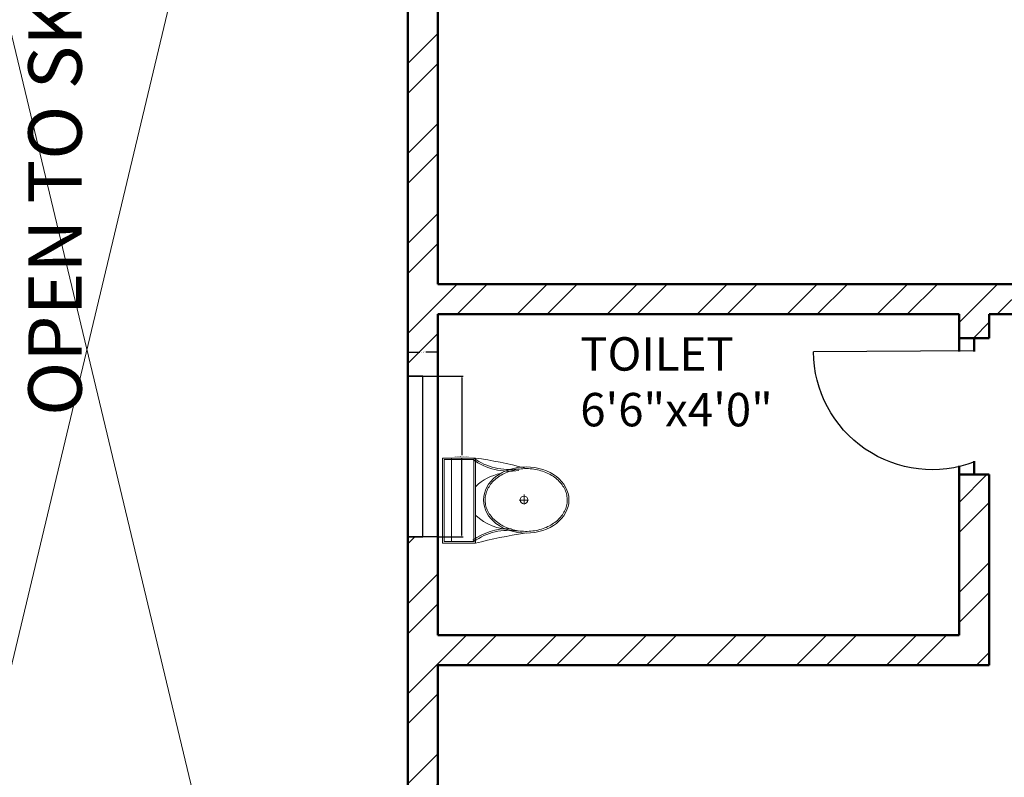
# Model space of a CAD drawing. Units: inches. Extents: x 1901 to 2863, y 888 to 2433.
# Tile 71 of 91: x 2381 to 2529, y 2009 to 2123. Entities that reach past the tile are written whole.
import ezdxf

# ---------------------------------------------------------------- set-up
doc = ezdxf.new("R2010")
doc.units = ezdxf.units.IN
for name, color, linetype, lineweight in [('A-ANNO-DIMS', 2, 'Continuous', 18), ('A-ANNO-SYMB', 8, 'Continuous', 13), ('A-AREA-IDEN', 7, 'Continuous', 18), ('A-DOOR', 4, 'Continuous', 25), ('A-FLOR-FIXT', 9, 'Continuous', 18), ('A-GLAZ', 3, 'Continuous', 25), ('A-WALL', 7, 'Continuous', 50), ('A-WALL-PATT', 8, 'Continuous', 13)]:
    doc.layers.add(name, color=color, linetype=linetype, lineweight=lineweight)
doc.styles.get("Standard").update_dxf_attribs({"font": 'arial.ttf'})
doc.dimstyles.get("Standard").update_dxf_attribs({"dimtxt": 0.18, "dimasz": 0.18, "dimexe": 0.18, "dimexo": 0.0625, "dimgap": 0.09, "dimtad": 0, "dimtih": 1, "dimtoh": 1, "dimdec": 4, "dimzin": 0, "dimdsep": 46, "dimtxsty": 'Standard', "dimcen": 0.09, "dimadec": 0, "dimazin": 0, "dimtfac": 1, "dimtdec": 4, "dimtofl": 0, "dimtmove": 0, "dimatfit": 3, "dimfxl": 1, "dimtolj": 1, "dimtzin": 0, "dimarcsym": 0})

# ---------------------------------------------------------------- blocks, each defined once
blk = doc.blocks.new('A$C31115884')
for p, q in [((283.1, 497.7), (223.4, 497.7)), ((257.5, 466.4), (257.5, 523.2)), ((0, 200), (0, 0)), ((520, 200), (0, 200)), ((10, 190), (10, 10)), ((510, 190), (10, 190)), ((510, 10), (510, 190)), ((520, 0), (520, 200)), ((510, 54.5), (0, 54.5)), ((10, 10), (510, 10)), ((0, 0), (520, 0))]:
    blk.add_line(p, q)
blk.add_circle((255.6, 496.4), 23.6)
for centre, radius, start, end in [((2777.7, -204.6), 2807, 165.4549, 171.71327), ((3237, 905), 2807, 188.28673, 194.5451), ((-294.5, 403.3), 364.7, 324.20913, 9.34987), ((-294.5, 403.3), 374.7, 324.20913, 9.34987), ((805.8, 403.3), 364.7, 170.65013, 215.79087), ((139.5, 406.2), 293.5, 315.84364, 2.65635), ((805.8, 403.3), 374.7, 179.20365, 215.79087), ((383.6, 406.2), 293.5, 190.27735, 224.15636)]:
    blk.add_arc(centre, radius, start, end)
blk.add_ellipse((256.2, 509.9), major_axis=(0, -260.7), ratio=0.772727)
blk.add_open_spline([(256.2, 259.2), (263.1, 259.2), (270, 259.7), (287.8, 262.3), (298.7, 265.1), (319.9, 273.1), (330.2, 278.4), (350.1, 291.1), (359.7, 298.7), (377.7, 315.9), (386.2, 325.5), (401.7, 346.6), (408.8, 358.1), (421.3, 382.5), (426.8, 395.5), (435.9, 422.4), (439.5, 436.4), (444.8, 465.1), (446.5, 479.7), (447.9, 509.2), (447.6, 524), (445, 553.3), (442.7, 567.8), (436.3, 596), (432.1, 609.7), (421.9, 636), (416, 648.6), (402.5, 672.1), (395, 683), (378.6, 703), (369.8, 712.1), (351.1, 728), (341.3, 734.8), (320.9, 746.2), (310.4, 750.7), (288.9, 757.3), (278, 759.4), (256, 761), (245, 760.6), (223.1, 757.2), (212.3, 754.3), (191.1, 746.1), (180.8, 740.7), (160.9, 727.8), (151.4, 720.1), (133.5, 702.7), (125.1, 693), (109.6, 671.7), (102.6, 660.2), (90.2, 635.7), (84.9, 622.7), (76, 595.6), (72.4, 581.6), (67.2, 552.9), (65.6, 538.2), (64.4, 508.8), (64.8, 494), (67.5, 464.7), (69.9, 450.2), (76.6, 422), (80.8, 408.3), (91.1, 382.2), (97.2, 369.7), (110.8, 346.3), (118.4, 335.4), (134.8, 315.6), (143.7, 306.7), (162.4, 290.9), (172.3, 284.2), (192.8, 273), (203.3, 268.6), (224.8, 262.2), (235.8, 260.2), (249.9, 259.3), (253, 259.2), (256.2, 259.2)], degree=3, knots=[0, 0, 0, 0, 0.110105, 0.110105, 0.285049, 0.285049, 0.459994, 0.459994, 0.634938, 0.634938, 0.809882, 0.809882, 0.984827, 0.984827, 1.159771, 1.159771, 1.334715, 1.334715, 1.50966, 1.50966, 1.684604, 1.684604, 1.859549, 1.859549, 2.034493, 2.034493, 2.209437, 2.209437, 2.384382, 2.384382, 2.559326, 2.559326, 2.73427, 2.73427, 2.909215, 2.909215, 3.084159, 3.084159, 3.259103, 3.259103, 3.434048, 3.434048, 3.608992, 3.608992, 3.783936, 3.783936, 3.958881, 3.958881, 4.133825, 4.133825, 4.30877, 4.30877, 4.483714, 4.483714, 4.658658, 4.658658, 4.833603, 4.833603, 5.008547, 5.008547, 5.183491, 5.183491, 5.358436, 5.358436, 5.53338, 5.53338, 5.708324, 5.708324, 5.883269, 5.883269, 6.058213, 6.058213, 6.233158, 6.233158, 6.283185, 6.283185, 6.283185, 6.283185])
blk = doc.blocks.new('WIN-24-3')
for p, q in [((0, 0), (0, 4.5)), ((0, 4.5), (0, 2.25)), ((24, 2.25), (24, 4.5)), ((24, 4.5), (24, 0)), ((0, 2.25), (24, 2.25))]:
    blk.add_line(p, q)
blk = doc.blocks.new('DOOR-18')
blk.add_line((23.98, -0.01), (-0.02, -0.01))
blk.add_arc((17.74, -0.01), 17.76, 69.4255, 180)
blk = doc.blocks.new('*D25')
at = {"layer": 'A-ANNO-DIMS', "color": 0, "lineweight": -2, "transparency": 16777216}
for p, q in [((2443.99, 2069.35), (2447.71, 2069.35)), ((2447.53, 2069.17), (2447.53, 2057.53)), ((2447.53, 2045.53), (2447.53, 2057.17)), ((2443.99, 2045.35), (2447.71, 2045.35))]:
    blk.add_line(p, q, dxfattribs=at)
at = {"layer": 'A-ANNO-DIMS', "color": 0, "transparency": 16777216}
for points in [[(2447.5, 2069.17), (2447.56, 2069.17), (2447.53, 2069.35)], [(2447.5, 2045.53), (2447.56, 2045.53), (2447.53, 2045.35)]]:
    blk.add_solid(points, dxfattribs=at)
at = {"layer": 'Defpoints', "color": 0, "transparency": 16777216}
for p in [(2443.93, 2069.35), (2447.53, 2069.35), (2443.93, 2045.35)]:
    blk.add_point(p, dxfattribs=at)
at = {"layer": 'A-ANNO-DIMS', "color": 0, "transparency": 16777216, "insert": (2447.53, 2057.35), "char_height": 0.18, "attachment_point": 5}
blk.add_mtext('\\A1;WINDOW W4 24 TYP.', dxfattribs=at)
blk = doc.blocks.new('*D26')
at = {"layer": 'A-ANNO-DIMS', "color": 0, "lineweight": -2, "transparency": 16777216}
for p, q in [((2439.43, 2069.41), (2439.43, 2073.13)), ((2439.61, 2072.95), (2441.22, 2072.95)), ((2443.75, 2072.95), (2442.13, 2072.95)), ((2443.93, 2069.41), (2443.93, 2073.13))]:
    blk.add_line(p, q, dxfattribs=at)
at = {"layer": 'A-ANNO-DIMS', "color": 0, "transparency": 16777216}
for points in [[(2439.61, 2072.98), (2439.61, 2072.92), (2439.43, 2072.95)], [(2443.75, 2072.98), (2443.75, 2072.92), (2443.93, 2072.95)]]:
    blk.add_solid(points, dxfattribs=at)
at = {"layer": 'Defpoints', "color": 0, "transparency": 16777216}
for p in [(2439.43, 2072.95), (2439.43, 2069.35), (2443.93, 2069.35)]:
    blk.add_point(p, dxfattribs=at)
at = {"layer": 'A-ANNO-DIMS', "color": 0, "transparency": 16777216, "insert": (2441.68, 2072.95), "char_height": 0.18, "attachment_point": 5}
blk.add_mtext('\\A1;5 TYP.', dxfattribs=at)

msp = doc.modelspace()

# ---------------------------------------------------------------- hatches: boundary and pattern name
at = {"layer": 'A-WALL-PATT'}
h = msp.add_hatch(dxfattribs=at)
h.set_pattern_fill('ANSI32', color=256)
h.paths.add_polyline_path([(2192.5, 2274.13), (2141.26, 2274.13), (2141.26, 2269.63), (2192.5, 2269.63)])
h.paths.add_polyline_path([(2259.93, 2274.13), (2216.5, 2274.13), (2216.5, 2269.63), (2255.43, 2269.63), (2255.43, 2214.63), (2250.81, 2214.63), (2250.81, 2210.13), (2259.93, 2210.13), (2259.93, 2215.13), (2271.76, 2215.13), (2271.76, 2217.38), (2271.76, 2219.63), (2259.93, 2219.63)])
h.paths.add_polyline_path([(2171.43, 2269.63), (2166.93, 2269.63), (2166.93, 2219.63), (2121.24, 2219.63), (2121.24, 2215.13), (2166.93, 2215.13), (2166.93, 2083.13), (2161.81, 2083.13), (2161.81, 2078.63), (2171.43, 2078.63), (2177, 2078.63), (2177, 2080.88), (2177, 2083.13), (2171.43, 2083.13), (2171.43, 2210.13), (2230.91, 2210.13), (2230.91, 2212.38), (2230.91, 2214.63), (2171.43, 2214.63)])
h.paths.add_polyline_path([(2117.26, 2274.13), (2089.43, 2274.13), (2089.43, 2219.63), (2081.14, 2219.63), (2081.14, 2215.13), (2089.43, 2215.13), (2098, 2215.13), (2098, 2217.38), (2098, 2219.63), (2093.93, 2219.63), (2093.93, 2269.63), (2117.26, 2269.63), (2117.26, 2271.88)])
h.paths.add_polyline_path([(2343.43, 2219.63), (2329.29, 2219.63), (2329.29, 2215.13), (2338.93, 2215.13), (2338.93, 2184.74), (2343.43, 2184.74)])
h.paths.add_polyline_path([(2338.93, 2083.13), (2329.29, 2083.13), (2208.97, 2083.13), (2208.97, 2078.63), (2338.93, 2078.63)])
h.paths.add_polyline_path([(2343.43, 2136.74), (2338.93, 2136.74), (2338.93, 1872.63), (2343.43, 1872.63)])
h.paths.add_polyline_path([(2343.43, 1863.63), (2397.68, 1863.63), (2397.68, 1821.63), (2384.14, 1821.63), (2384.14, 1812.63), (2418.33, 1812.63), (2418.33, 1817.13), (2418.33, 1821.63), (2406.68, 1821.63), (2406.68, 1863.63), (2459.5, 1863.63), (2459.5, 1821.63), (2447.14, 1821.63), (2447.14, 1812.63), (2459.5, 1812.63), (2468.5, 1812.63), (2468.5, 1872.63), (2394.43, 1872.63), (2334.43, 1872.63), (2334.43, 1812.63), (2343.43, 1812.63), (2353.25, 1812.63), (2353.25, 1821.63), (2343.43, 1821.63)])
h.paths.add_polyline_path([(2510.01, 1872.63), (2468.5, 1872.63), (2468.5, 1868.13), (2510.01, 1868.13)])
h.paths.add_polyline_path([(2514.01, 1817.13), (2468.5, 1817.13), (2468.5, 1812.63), (2482.11, 1812.63), (2482.11, 1800.61), (2486.61, 1800.61), (2486.61, 1812.63), (2514.01, 1812.63)])
h.paths.add_polyline_path([(2299.25, 1814.88), (2299.25, 1817.13), (2295.93, 1817.13), (2295.93, 1854.17), (2293.68, 1854.17), (2291.43, 1854.17), (2291.43, 1817.13), (2266.11, 1817.13), (2266.11, 1812.63), (2299.25, 1812.63)])
h.paths.add_polyline_path([(2218.11, 1817.13), (2206.46, 1817.13), (2171.43, 1817.13), (2171.43, 1949.13), (2190.1, 1949.13), (2190.1, 1953.63), (2163.47, 1953.63), (2163.47, 1949.13), (2166.93, 1949.13), (2166.93, 1817.13), (2114.3, 1817.13), (2114.3, 1812.63), (2218.11, 1812.63)])
h.paths.add_polyline_path([(2029.43, 1970.92), (2024.93, 1970.92), (2024.93, 1912.72), (2029.43, 1912.72)])
h.paths.add_polyline_path([(2132.3, 1953.63), (2113.93, 1953.63), (2113.93, 1975.89), (2111.68, 1975.89), (2109.43, 1975.89), (2109.43, 1953.63), (2029.43, 1953.63), (2029.43, 1949.13), (2132.3, 1949.13)])
h.paths.add_polyline_path([(2029.43, 1853.61), (2029.31, 1853.61), (2029.31, 1853.61), (2029.43, 1853.61), (2029.43, 1864.72), (2024.93, 1864.72), (2024.93, 1812.63), (2066.3, 1812.63), (2066.3, 1814.88), (2066.3, 1817.13), (2029.43, 1817.13)])
h.paths.add_polyline_path([(2122.93, 2010.09), (2120.68, 2010.09), (2118.43, 2010.09), (2118.43, 2006.13), (2029.43, 2006.13), (2029.43, 2001.63), (2109.43, 2001.63), (2109.43, 1998.04), (2113.93, 1998.04), (2113.93, 2001.63), (2122.93, 2001.63)])
h.paths.add_polyline_path([(2029.43, 2031.38), (2024.93, 2031.38), (2024.93, 1994.92), (2027.18, 1994.92), (2029.43, 1994.92)])
h.paths.add_polyline_path([(2029.43, 2136.74), (2024.93, 2136.74), (2024.93, 2067.38), (2027.18, 2067.38), (2029.43, 2067.38)])
h.paths.add_polyline_path([(2125.62, 2083.13), (2029.43, 2083.13), (2029.43, 2078.63), (2118.43, 2078.63), (2118.43, 2030.71), (2122.93, 2030.71), (2122.93, 2078.63), (2125.62, 2078.63)])
h.paths.add_polyline_path([(2029.43, 2215.13), (2040.47, 2215.13), (2040.47, 2217.38), (2040.47, 2219.63), (2024.93, 2219.63), (2024.93, 2184.74), (2029.43, 2184.74), (2029.43, 2187.78)])
h.paths.add_polyline_path([(2686.43, 2274.13), (2659.28, 2274.13), (2659.28, 2269.63), (2681.93, 2269.63), (2681.93, 2219.63), (2676.82, 2219.63), (2676.82, 2215.13), (2681.93, 2215.13), (2697.01, 2215.13), (2697.01, 2217.38), (2697.01, 2219.63), (2686.43, 2219.63)])
h.paths.add_polyline_path([(2609.93, 2269.63), (2635.28, 2269.63), (2635.28, 2274.13), (2571.43, 2274.13), (2571.43, 2269.63), (2605.43, 2269.63), (2605.43, 2214.63), (2549.1, 2214.63), (2549.1, 2210.13), (2605.43, 2210.13), (2605.43, 2083.13), (2601.01, 2083.13), (2601.01, 2080.88), (2601.01, 2078.63), (2609.93, 2078.63), (2616.16, 2078.63), (2616.16, 2080.88), (2616.16, 2083.13), (2609.93, 2083.13), (2609.93, 2215.13), (2651.46, 2215.13), (2651.46, 2217.38), (2651.46, 2219.63), (2609.93, 2219.63)])
h.paths.add_polyline_path([(2521.43, 2269.63), (2547.43, 2269.63), (2547.43, 2271.88), (2547.43, 2274.13), (2516.93, 2274.13), (2516.93, 2219.63), (2506.41, 2219.63), (2506.41, 2215.13), (2516.93, 2215.13), (2516.93, 2210.13), (2525.4, 2210.13), (2525.4, 2212.38), (2525.4, 2214.63), (2521.43, 2214.63)])
h.paths.add_polyline_path([(2456.01, 2219.63), (2439.43, 2219.63), (2439.43, 2187.89), (2443.93, 2187.89), (2443.93, 2215.13), (2456.01, 2215.13)])
h.paths.add_polyline_path([(2752.93, 2219.63), (2739.48, 2219.63), (2739.48, 2215.13), (2748.43, 2215.13), (2748.43, 2187.89), (2752.93, 2187.89)])
h.paths.add_polyline_path([(2752.93, 2139.89), (2748.43, 2139.89), (2748.43, 2083.13), (2648.42, 2083.13), (2648.42, 2078.63), (2654.93, 2078.63), (2654.93, 2039.44), (2659.43, 2039.44), (2659.43, 2078.63), (2748.43, 2078.63), (2748.43, 2063.43), (2752.93, 2063.43)])
h.paths.add_polyline_path([(2752.93, 2010.63), (2659.43, 2010.63), (2659.43, 2015.65), (2654.93, 2015.65), (2654.93, 2010.63), (2605.43, 2010.63), (2605.43, 1920.97), (2609.93, 1920.97), (2609.93, 2006.13), (2748.43, 2006.13), (2748.43, 1982.47), (2752.93, 1982.47)])
h.paths.add_polyline_path([(2752.93, 2027.43), (2748.43, 2027.43), (2748.43, 2010.63), (2752.93, 2010.63)])
h.paths.add_polyline_path([(2748.43, 1886.13), (2609.93, 1886.13), (2609.93, 1889.72), (2605.43, 1889.72), (2605.43, 1861.26), (2609.93, 1861.26), (2609.93, 1881.63), (2748.43, 1881.63)])
h.paths.add_polyline_path([(2456.86, 2228.83), (2498.4, 2228.83), (2498.4, 2247.49), (2456.86, 2247.49)], flags=9)
h.paths.add_polyline_path([(2038.6, 2237.42), (2080.17, 2237.42), (2080.17, 2256.08), (2038.6, 2256.08)], flags=9)
h.paths.add_polyline_path([(2292.01, 1062.39), (2539.93, 1062.39), (2539.93, 1099.49), (2292.01, 1099.49)], flags=9)
h.paths.add_polyline_path([(2424.91, 1832.25), (2448.51, 1832.25), (2448.51, 1846.68), (2424.91, 1846.68)], flags=25)
h.paths.add_polyline_path([(2359.08, 1832.25), (2382.68, 1832.25), (2382.68, 1846.68), (2359.08, 1846.68)], flags=25)
h.paths.add_polyline_path([(2352.9, 1684.8), (2367.54, 1684.8), (2367.54, 1697.17), (2352.9, 1697.17)], flags=9)
h.paths.add_polyline_path([(2079.29, 1755.83), (2169.02, 1755.83), (2169.02, 1774.37), (2079.29, 1774.37)], flags=9)
h.paths.add_polyline_path([(2404.09, 1373.86), (2404.09, 1463.59), (2385.54, 1463.59), (2385.54, 1373.86)], flags=9)
h.paths.add_polyline_path([(2268.09, 2236.37), (2309.64, 2236.37), (2309.64, 2255.03), (2268.09, 2255.03)], flags=9)
h.paths.add_polyline_path([(2575.96, 1700.95), (2665.7, 1700.95), (2665.7, 1719.5), (2575.96, 1719.5)], flags=9)
h.paths.add_polyline_path([(2302.96, 1878.47), (2329.52, 1878.47), (2329.52, 1888.78), (2302.96, 1888.78)], flags=9)
h.paths.add_polyline_path([(2097.42, 2240.58), (2126.57, 2240.58), (2126.57, 2259.23), (2097.42, 2259.23)], flags=9)
h.paths.add_polyline_path([(2208.72, 2246.12), (2237.88, 2246.12), (2237.88, 2264.78), (2208.72, 2264.78)], flags=9)
h.paths.add_polyline_path([(2038.15, 1925.96), (2076.99, 1925.96), (2076.99, 1944.62), (2038.15, 1944.62)], flags=9)
h.paths.add_polyline_path([(2239.14, 1926.67), (2288.46, 1926.67), (2288.46, 1945.33), (2239.14, 1945.33)], flags=9)
h.paths.add_polyline_path([(2175.43, 2007.33), (2212.36, 2007.33), (2212.36, 2025.99), (2175.43, 2025.99)], flags=9)
h.paths.add_polyline_path([(2225.03, 2091.79), (2263.87, 2091.79), (2263.87, 2110.45), (2225.03, 2110.45)], flags=9)
h.paths.add_polyline_path([(2035.4, 2098.48), (2074.24, 2098.48), (2074.24, 2117.14), (2035.4, 2117.14)], flags=9)
h.paths.add_polyline_path([(2050.1, 2029.21), (2083.26, 2029.21), (2083.26, 2047.87), (2050.1, 2047.87)], flags=9)
h.paths.add_polyline_path([(2069.68, 1956.72), (2098.83, 1956.72), (2098.83, 1975.38), (2069.68, 1975.38)], flags=25)
h.paths.add_polyline_path([(2328.62, 1753.34), (2361.66, 1753.34), (2361.66, 1771.99), (2328.62, 1771.99)], flags=9)
h.paths.add_polyline_path([(2395.16, 2060.89), (2395.16, 2140.65), (2378.68, 2140.65), (2378.68, 2060.89)], flags=9)
h.paths.add_polyline_path([(2463.73, 2059.02), (2492.89, 2059.02), (2492.89, 2077.68), (2463.73, 2077.68)], flags=9)
h.paths.add_polyline_path([(2458.03, 2181.54), (2496.87, 2181.54), (2496.87, 2200.19), (2458.03, 2200.19)], flags=9)
h.paths.add_polyline_path([(2527.58, 2243.07), (2556.73, 2243.07), (2556.73, 2261.73), (2527.58, 2261.73)], flags=9)
h.paths.add_polyline_path([(2694.46, 2232.77), (2736.03, 2232.77), (2736.03, 2251.42), (2694.46, 2251.42)], flags=9)
h.paths.add_polyline_path([(2637.82, 2249.22), (2666.98, 2249.22), (2666.98, 2267.88), (2637.82, 2267.88)], flags=9)
h.paths.add_polyline_path([(2623.69, 2183.54), (2662.53, 2183.54), (2662.53, 2202.2), (2623.69, 2202.2)], flags=9)
h.paths.add_polyline_path([(2691.97, 2021.5), (2725.12, 2021.5), (2725.12, 2040.16), (2691.97, 2040.16)], flags=9)
h.paths.add_polyline_path([(2621.04, 1975.91), (2662.34, 1975.91), (2662.34, 1994.57), (2621.04, 1994.57)], flags=25)
h.paths.add_polyline_path([(2479.03, 1927.62), (2519.84, 1927.62), (2519.84, 1946.28), (2479.03, 1946.28)], flags=9)
h.paths.add_polyline_path([(2670.94, 1849.08), (2716.01, 1849.08), (2716.01, 1867.73), (2670.94, 1867.73)], flags=9)
h.paths.add_polyline_path([(2523.61, 1782.96), (2550.17, 1782.96), (2550.17, 1793.26), (2523.61, 1793.26)], flags=9)
h.paths.add_polyline_path([(2450.84, 1207.33), (2492.39, 1207.33), (2492.39, 1225.99), (2450.84, 1225.99)], flags=9)
h.paths.add_polyline_path([(2527.75, 1203.84), (2556.91, 1203.84), (2556.91, 1222.5), (2527.75, 1222.5)], flags=9)
h.paths.add_polyline_path([(2639.11, 1207.2), (2668.27, 1207.2), (2668.27, 1225.86), (2639.11, 1225.86)], flags=9)
h.paths.add_polyline_path([(2692.59, 1218.97), (2734.17, 1218.97), (2734.17, 1237.62), (2692.59, 1237.62)], flags=9)
h.paths.add_polyline_path([(2669.27, 1366.33), (2708.11, 1366.33), (2708.11, 1384.99), (2669.27, 1384.99)], flags=9)
h.paths.add_polyline_path([(2463.31, 1358.03), (2502.15, 1358.03), (2502.15, 1376.69), (2463.31, 1376.69)], flags=9)
h.paths.add_polyline_path([(2494.72, 1449.96), (2531.65, 1449.96), (2531.65, 1468.62), (2494.72, 1468.62)], flags=9)
h.paths.add_polyline_path([(2675.57, 1422.16), (2708.72, 1422.16), (2708.72, 1440.81), (2675.57, 1440.81)], flags=9)
h.paths.add_polyline_path([(2685.63, 1493.89), (2714.79, 1493.89), (2714.79, 1512.55), (2685.63, 1512.55)], flags=9)
h.paths.add_polyline_path([(2686.8, 1529.91), (2725.65, 1529.91), (2725.65, 1548.57), (2686.8, 1548.57)], flags=9)
h.paths.add_polyline_path([(2503.65, 1537.99), (2552.97, 1537.99), (2552.97, 1556.65), (2503.65, 1556.65)], flags=9)
h.paths.add_polyline_path([(2291.71, 1643.5), (2318.28, 1643.5), (2318.28, 1653.81), (2291.71, 1653.81)], flags=9)
h.paths.add_polyline_path([(2450.63, 1610.52), (2477.19, 1610.52), (2477.19, 1620.82), (2450.63, 1620.82)], flags=9)
h.paths.add_polyline_path([(2359.99, 1551.81), (2422.25, 1551.81), (2422.25, 1562.12), (2359.99, 1562.12)], flags=9)
h.paths.add_polyline_path([(2280.11, 1249.01), (2321.65, 1249.01), (2321.65, 1267.66), (2280.11, 1267.66)], flags=9)
h.paths.add_polyline_path([(2164.06, 1274.23), (2193.22, 1274.23), (2193.22, 1292.89), (2164.06, 1292.89)], flags=9)
h.paths.add_polyline_path([(2118.21, 1277.69), (2151.25, 1277.69), (2151.25, 1296.35), (2118.21, 1296.35)], flags=9)
h.paths.add_polyline_path([(2031.95, 1268.53), (2073.52, 1268.53), (2073.52, 1287.19), (2031.95, 1287.19)], flags=9)
h.paths.add_polyline_path([(2050.2, 1409.08), (2089.04, 1409.08), (2089.04, 1427.74), (2050.2, 1427.74)], flags=9)
h.paths.add_polyline_path([(2243.74, 1421.03), (2282.58, 1421.03), (2282.58, 1439.69), (2243.74, 1439.69)], flags=9)
h.paths.add_polyline_path([(2190.75, 1509.77), (2231.56, 1509.77), (2231.56, 1528.43), (2190.75, 1528.43)], flags=9)
h.paths.add_polyline_path([(2058.39, 1475.42), (2091.55, 1475.42), (2091.55, 1494.07), (2058.39, 1494.07)], flags=9)
h.paths.add_polyline_path([(2062.45, 1553.09), (2091.6, 1553.09), (2091.6, 1571.75), (2062.45, 1571.75)], flags=9)
h.paths.add_polyline_path([(2219.52, 1590.37), (2266.15, 1590.37), (2266.15, 1609.02), (2219.52, 1609.02)], flags=9)
h.paths.add_polyline_path([(2041.07, 1584.19), (2079.91, 1584.19), (2079.91, 1602.85), (2041.07, 1602.85)], flags=9)
h = msp.add_hatch(dxfattribs=at)
h.set_pattern_fill('ANSI32', color=256)
h.paths.add_polyline_path([(2443.93, 2139.89), (2439.43, 2139.89), (2439.43, 2069.35), (2441.68, 2069.35), (2443.93, 2069.35), (2443.93, 2078.63), (2521.93, 2078.63), (2521.93, 2075.07), (2524.18, 2075.07), (2526.43, 2075.07), (2526.43, 2078.63), (2571.75, 2078.63), (2571.75, 2080.88), (2571.75, 2083.13), (2443.93, 2083.13)])
h.paths.add_polyline_path([(2526.43, 2054.63), (2524.18, 2054.63), (2521.93, 2054.63), (2521.93, 2030.63), (2443.93, 2030.63), (2443.93, 2045.35), (2439.43, 2045.35), (2439.43, 1983.87), (2443.93, 1983.87), (2443.93, 2026.13), (2521.93, 2026.13), (2526.43, 2026.13)])
h.paths.add_polyline_path([(2443.93, 1923.87), (2439.43, 1923.87), (2439.43, 1872.63), (2443.93, 1872.63)])
h.paths.add_polyline_path([(2636.23, 1766.13), (2609.93, 1766.13), (2609.93, 1779.79), (2605.43, 1779.79), (2605.43, 1766.13), (2486.61, 1766.13), (2486.61, 1770.67), (2482.11, 1770.67), (2482.11, 1766.13), (2482.11, 1761.63), (2636.23, 1761.63), (2636.23, 1763.88)])
h.paths.add_polyline_path([(2519.54, 1663.38), (2519.54, 1665.63), (2494.93, 1665.63), (2481.83, 1665.63), (2481.83, 1663.38), (2481.83, 1661.13), (2490.43, 1661.13), (2490.43, 1640.16), (2494.93, 1640.16), (2494.93, 1661.13), (2519.54, 1661.13)])
h.paths.add_polyline_path([(2443.93, 1712.13), (2443.93, 1716.63), (2414.46, 1716.63), (2414.46, 1712.13), (2439.43, 1712.13), (2439.43, 1545.51), (2443.93, 1545.51), (2443.93, 1661.13), (2448.47, 1661.13), (2448.47, 1665.63), (2443.93, 1665.63)])
h.paths.add_polyline_path([(2343.43, 1712.13), (2365.52, 1712.13), (2365.52, 1714.38), (2365.52, 1716.63), (2333.87, 1716.63), (2333.87, 1714.38), (2333.87, 1712.13), (2338.93, 1712.13), (2338.93, 1575.63), (2338.93, 1545.51), (2343.43, 1545.51), (2343.43, 1547.51), (2343.43, 1580.13)])
h.paths.add_polyline_path([(2752.93, 1665.63), (2579.54, 1665.63), (2579.54, 1661.13), (2615.93, 1661.13), (2615.93, 1529.13), (2598.93, 1529.13), (2598.93, 1524.63), (2623.13, 1524.63), (2623.13, 1526.88), (2623.13, 1529.13), (2620.43, 1529.13), (2620.43, 1661.13), (2748.43, 1661.13), (2748.43, 1633.5), (2752.93, 1633.5)])
h.paths.add_polyline_path([(2752.93, 1419.93), (2748.43, 1419.93), (2748.43, 1400.13), (2659.43, 1400.13), (2659.43, 1444.33), (2657.18, 1444.33), (2654.93, 1444.33), (2654.93, 1400.13), (2643.65, 1400.13), (2643.65, 1395.63), (2748.43, 1395.63), (2748.43, 1364.04), (2752.93, 1364.04)])
h.paths.add_polyline_path([(2752.93, 1492.88), (2748.43, 1492.88), (2748.43, 1476.63), (2667.43, 1476.63), (2667.43, 1479.71), (2665.18, 1479.71), (2662.93, 1479.71), (2662.93, 1476.63), (2654.93, 1476.63), (2654.93, 1469.54), (2659.43, 1469.54), (2659.43, 1472.13), (2748.43, 1472.13), (2748.43, 1455.93), (2752.93, 1455.93)])
h.paths.add_polyline_path([(2752.93, 1304.04), (2748.43, 1304.04), (2748.43, 1263.63), (2738.66, 1263.63), (2738.66, 1259.13), (2752.93, 1259.13)])
h.paths.add_polyline_path([(2685.93, 1259.13), (2695.49, 1259.13), (2695.49, 1261.38), (2695.49, 1263.63), (2677.84, 1263.63), (2677.84, 1261.38), (2677.84, 1259.13), (2681.43, 1259.13), (2681.43, 1203.63), (2653.28, 1203.63), (2653.28, 1199.13), (2685.93, 1199.13), (2685.93, 1203.63)])
h.paths.add_polyline_path([(2609.43, 1395.63), (2611.85, 1395.63), (2611.85, 1400.13), (2598.89, 1400.13), (2598.89, 1397.88), (2598.89, 1395.63), (2604.93, 1395.63), (2604.93, 1268.13), (2554.73, 1268.13), (2554.73, 1265.88), (2554.73, 1263.63), (2604.93, 1263.63), (2604.93, 1203.63), (2571.31, 1203.63), (2571.31, 1199.13), (2604.93, 1199.13), (2629.28, 1199.13), (2629.28, 1201.38), (2629.28, 1203.63), (2609.43, 1203.63), (2609.43, 1258.63), (2609.43, 1259.13), (2654.8, 1259.13), (2654.8, 1263.63), (2609.43, 1263.63)])
h.paths.add_polyline_path([(2443.93, 1304.04), (2439.43, 1304.04), (2439.43, 1259.13), (2443.93, 1259.13), (2456.16, 1259.13), (2456.16, 1261.38), (2456.16, 1263.63), (2443.93, 1263.63)])
h.paths.add_polyline_path([(2525.43, 1263.63), (2531.78, 1263.63), (2531.78, 1268.13), (2520.93, 1268.13), (2520.93, 1263.63), (2511.41, 1263.63), (2511.41, 1259.13), (2520.93, 1259.13), (2520.93, 1199.13), (2547.31, 1199.13), (2547.31, 1201.38), (2547.31, 1203.63), (2525.43, 1203.63)])
h.paths.add_polyline_path([(2443.93, 1434.84), (2439.43, 1434.84), (2439.43, 1364.04), (2441.68, 1364.04), (2443.93, 1364.04)])
h.paths.add_polyline_path([(2567.13, 1400.13), (2443.93, 1400.13), (2443.93, 1395.63), (2567.13, 1395.63)])
h.paths.add_polyline_path([(2443.93, 1545.51), (2439.43, 1545.51), (2439.43, 1494.84), (2443.93, 1494.84)])
h.paths.add_polyline_path([(2494.93, 1553.35), (2492.68, 1553.35), (2490.43, 1553.35), (2490.43, 1524.63), (2494.93, 1524.63), (2525.94, 1524.63), (2525.94, 1526.88), (2525.94, 1529.13), (2494.93, 1529.13)])
h.paths.add_polyline_path([(2752.93, 1573.5), (2748.43, 1573.5), (2748.43, 1529.13), (2657.76, 1529.13), (2657.76, 1524.63), (2662.93, 1524.63), (2662.93, 1498.63), (2667.43, 1498.63), (2667.43, 1524.63), (2748.43, 1524.63), (2748.43, 1516.88), (2752.93, 1516.88)])
h.paths.add_polyline_path([(2038.6, 2237.42), (2080.17, 2237.42), (2080.17, 2256.08), (2038.6, 2256.08)], flags=9)
h.paths.add_polyline_path([(2292.01, 1062.39), (2539.93, 1062.39), (2539.93, 1099.49), (2292.01, 1099.49)], flags=9)
h.paths.add_polyline_path([(2424.91, 1832.25), (2448.51, 1832.25), (2448.51, 1846.68), (2424.91, 1846.68)], flags=9)
h.paths.add_polyline_path([(2359.08, 1832.25), (2382.68, 1832.25), (2382.68, 1846.68), (2359.08, 1846.68)], flags=9)
h.paths.add_polyline_path([(2352.9, 1684.8), (2367.54, 1684.8), (2367.54, 1697.17), (2352.9, 1697.17)], flags=9)
h.paths.add_polyline_path([(2079.29, 1755.83), (2169.02, 1755.83), (2169.02, 1774.37), (2079.29, 1774.37)], flags=9)
h.paths.add_polyline_path([(2404.09, 1373.86), (2404.09, 1463.59), (2385.54, 1463.59), (2385.54, 1373.86)], flags=9)
h.paths.add_polyline_path([(2268.09, 2236.37), (2309.64, 2236.37), (2309.64, 2255.03), (2268.09, 2255.03)], flags=9)
h.paths.add_polyline_path([(2575.96, 1700.95), (2665.7, 1700.95), (2665.7, 1719.5), (2575.96, 1719.5)], flags=9)
h.paths.add_polyline_path([(2302.96, 1878.47), (2329.52, 1878.47), (2329.52, 1888.78), (2302.96, 1888.78)], flags=9)
h.paths.add_polyline_path([(2097.42, 2240.58), (2126.57, 2240.58), (2126.57, 2259.23), (2097.42, 2259.23)], flags=9)
h.paths.add_polyline_path([(2208.72, 2246.12), (2237.88, 2246.12), (2237.88, 2264.78), (2208.72, 2264.78)], flags=9)
h.paths.add_polyline_path([(2038.15, 1925.96), (2076.99, 1925.96), (2076.99, 1944.62), (2038.15, 1944.62)], flags=9)
h.paths.add_polyline_path([(2239.14, 1926.67), (2288.46, 1926.67), (2288.46, 1945.33), (2239.14, 1945.33)], flags=9)
h.paths.add_polyline_path([(2175.43, 2007.33), (2212.36, 2007.33), (2212.36, 2025.99), (2175.43, 2025.99)], flags=9)
h.paths.add_polyline_path([(2225.03, 2091.79), (2263.87, 2091.79), (2263.87, 2110.45), (2225.03, 2110.45)], flags=9)
h.paths.add_polyline_path([(2035.4, 2098.48), (2074.24, 2098.48), (2074.24, 2117.14), (2035.4, 2117.14)], flags=9)
h.paths.add_polyline_path([(2050.1, 2029.21), (2083.26, 2029.21), (2083.26, 2047.87), (2050.1, 2047.87)], flags=9)
h.paths.add_polyline_path([(2069.68, 1956.72), (2098.83, 1956.72), (2098.83, 1975.38), (2069.68, 1975.38)], flags=9)
h.paths.add_polyline_path([(2328.62, 1753.34), (2361.66, 1753.34), (2361.66, 1771.99), (2328.62, 1771.99)], flags=9)
h.paths.add_polyline_path([(2395.16, 2060.89), (2395.16, 2140.65), (2378.68, 2140.65), (2378.68, 2060.89)], flags=9)
h.paths.add_polyline_path([(2463.73, 2059.02), (2492.89, 2059.02), (2492.89, 2077.68), (2463.73, 2077.68)], flags=9)
h.paths.add_polyline_path([(2458.03, 2181.54), (2496.87, 2181.54), (2496.87, 2200.19), (2458.03, 2200.19)], flags=9)
h.paths.add_polyline_path([(2456.86, 2228.83), (2498.4, 2228.83), (2498.4, 2247.49), (2456.86, 2247.49)], flags=9)
h.paths.add_polyline_path([(2527.58, 2243.07), (2556.73, 2243.07), (2556.73, 2261.73), (2527.58, 2261.73)], flags=9)
h.paths.add_polyline_path([(2694.46, 2232.77), (2736.03, 2232.77), (2736.03, 2251.42), (2694.46, 2251.42)], flags=9)
h.paths.add_polyline_path([(2637.82, 2249.22), (2666.98, 2249.22), (2666.98, 2267.88), (2637.82, 2267.88)], flags=9)
h.paths.add_polyline_path([(2623.69, 2183.54), (2662.53, 2183.54), (2662.53, 2202.2), (2623.69, 2202.2)], flags=9)
h.paths.add_polyline_path([(2691.97, 2021.5), (2725.12, 2021.5), (2725.12, 2040.16), (2691.97, 2040.16)], flags=9)
h.paths.add_polyline_path([(2621.04, 1975.91), (2662.34, 1975.91), (2662.34, 1994.57), (2621.04, 1994.57)], flags=9)
h.paths.add_polyline_path([(2479.03, 1927.62), (2519.84, 1927.62), (2519.84, 1946.28), (2479.03, 1946.28)], flags=9)
h.paths.add_polyline_path([(2670.94, 1849.08), (2716.01, 1849.08), (2716.01, 1867.73), (2670.94, 1867.73)], flags=9)
h.paths.add_polyline_path([(2523.61, 1782.96), (2550.17, 1782.96), (2550.17, 1793.26), (2523.61, 1793.26)], flags=9)
h.paths.add_polyline_path([(2450.84, 1207.33), (2492.39, 1207.33), (2492.39, 1225.99), (2450.84, 1225.99)], flags=9)
h.paths.add_polyline_path([(2527.75, 1203.84), (2556.91, 1203.84), (2556.91, 1222.5), (2527.75, 1222.5)], flags=9)
h.paths.add_polyline_path([(2639.11, 1207.2), (2668.27, 1207.2), (2668.27, 1225.86), (2639.11, 1225.86)], flags=9)
h.paths.add_polyline_path([(2692.59, 1218.97), (2734.17, 1218.97), (2734.17, 1237.62), (2692.59, 1237.62)], flags=9)
h.paths.add_polyline_path([(2669.27, 1366.33), (2708.11, 1366.33), (2708.11, 1384.99), (2669.27, 1384.99)], flags=25)
h.paths.add_polyline_path([(2463.31, 1358.03), (2502.15, 1358.03), (2502.15, 1376.69), (2463.31, 1376.69)], flags=9)
h.paths.add_polyline_path([(2494.72, 1449.96), (2531.65, 1449.96), (2531.65, 1468.62), (2494.72, 1468.62)], flags=9)
h.paths.add_polyline_path([(2675.57, 1422.16), (2708.72, 1422.16), (2708.72, 1440.81), (2675.57, 1440.81)], flags=25)
h.paths.add_polyline_path([(2685.63, 1493.89), (2714.79, 1493.89), (2714.79, 1512.55), (2685.63, 1512.55)], flags=9)
h.paths.add_polyline_path([(2686.8, 1529.91), (2725.65, 1529.91), (2725.65, 1548.57), (2686.8, 1548.57)], flags=25)
h.paths.add_polyline_path([(2503.65, 1537.99), (2552.97, 1537.99), (2552.97, 1556.65), (2503.65, 1556.65)], flags=9)
h.paths.add_polyline_path([(2291.71, 1643.5), (2318.28, 1643.5), (2318.28, 1653.81), (2291.71, 1653.81)], flags=9)
h.paths.add_polyline_path([(2450.63, 1610.52), (2477.19, 1610.52), (2477.19, 1620.82), (2450.63, 1620.82)], flags=9)
h.paths.add_polyline_path([(2359.99, 1551.81), (2422.25, 1551.81), (2422.25, 1562.12), (2359.99, 1562.12)], flags=9)
h.paths.add_polyline_path([(2280.11, 1249.01), (2321.65, 1249.01), (2321.65, 1267.66), (2280.11, 1267.66)], flags=9)
h.paths.add_polyline_path([(2164.06, 1274.23), (2193.22, 1274.23), (2193.22, 1292.89), (2164.06, 1292.89)], flags=9)
h.paths.add_polyline_path([(2118.21, 1277.69), (2151.25, 1277.69), (2151.25, 1296.35), (2118.21, 1296.35)], flags=9)
h.paths.add_polyline_path([(2031.95, 1268.53), (2073.52, 1268.53), (2073.52, 1287.19), (2031.95, 1287.19)], flags=9)
h.paths.add_polyline_path([(2050.2, 1409.08), (2089.04, 1409.08), (2089.04, 1427.74), (2050.2, 1427.74)], flags=9)
h.paths.add_polyline_path([(2243.74, 1421.03), (2282.58, 1421.03), (2282.58, 1439.69), (2243.74, 1439.69)], flags=9)
h.paths.add_polyline_path([(2190.75, 1509.77), (2231.56, 1509.77), (2231.56, 1528.43), (2190.75, 1528.43)], flags=9)
h.paths.add_polyline_path([(2058.39, 1475.42), (2091.55, 1475.42), (2091.55, 1494.07), (2058.39, 1494.07)], flags=9)
h.paths.add_polyline_path([(2062.45, 1553.09), (2091.6, 1553.09), (2091.6, 1571.75), (2062.45, 1571.75)], flags=9)
h.paths.add_polyline_path([(2219.52, 1590.37), (2266.15, 1590.37), (2266.15, 1609.02), (2219.52, 1609.02)], flags=9)
h.paths.add_polyline_path([(2041.07, 1584.19), (2079.91, 1584.19), (2079.91, 1602.85), (2041.07, 1602.85)], flags=9)

# ---------------------------------------------------------------- linework, layer by layer
at = {"layer": 'A-ANNO-SYMB'}
for p, q in [((2343.43, 2274.13), (2439.43, 1872.63)), ((2343.43, 1872.63), (2439.43, 2274.13))]:
    msp.add_line(p, q, dxfattribs=at)
at = {"layer": 'A-WALL'}
for p, q in [((2439.43, 2219.63), (2439.43, 1872.63)), ((2443.93, 2215.13), (2443.93, 2083.13)), ((2443.93, 2083.13), (2573.05, 2083.13)), ((2506.41, 2083.13), (2516.93, 2083.13)), ((2443.93, 2078.63), (2521.93, 2078.63)), ((2443.93, 2078.63), (2443.93, 2030.63)), ((2521.93, 2073.07), (2521.93, 2078.63)), ((2526.43, 2078.63), (2526.43, 2075.07)), ((2526.43, 2078.63), (2571.75, 2078.63)), ((2526.43, 2075.07), (2521.93, 2075.07)), ((2521.93, 2075.07), (2524.18, 2075.07)), ((2524.18, 2075.07), (2524.18, 2073.07)), ((2521.93, 2030.63), (2521.93, 2055.93)), ((2524.18, 2054.63), (2524.18, 2056.63)), ((2521.93, 2054.63), (2526.43, 2054.63)), ((2526.43, 2054.63), (2524.18, 2054.63)), ((2526.43, 2054.63), (2526.43, 2026.13)), ((2443.93, 2030.63), (2521.93, 2030.63)), ((2443.93, 2026.13), (2526.43, 2026.13)), ((2443.93, 2026.13), (2443.93, 1872.63)), ((2443.93, 2026.13), (2521.93, 2026.13))]:
    msp.add_line(p, q, dxfattribs=at)

# ---------------------------------------------------------------- block references
at = {"layer": 'A-DOOR', "extrusion": (0, 0, -1), "zscale": -1, "rotation": 179.6024214091829}
msp.add_blockref('DOOR-18', (-2500.15, 2073), dxfattribs=at)
at = {"layer": 'A-FLOR-FIXT', "xscale": 0.0245149588751191, "yscale": 0.0245149588751191, "zscale": 0.0245149588751191, "rotation": 270}
msp.add_blockref('A$C31115884', (2444.65, 2057.12), dxfattribs=at)
at = {"layer": 'A-GLAZ', "rotation": 89.99999999999815}
msp.add_blockref('WIN-24-3', (2443.93, 2045.35), dxfattribs=at)

# ---------------------------------------------------------------- texts
at = {"layer": 'A-AREA-IDEN', "insert": (2382.65, 2063.43), "char_height": 8, "attachment_point": 1, "rotation": 90}
msp.add_mtext_dynamic_manual_height_columns('OPEN TO SKY', width=370.2743, gutter_width=12.5, heights=[0], dxfattribs=at)
at = {"layer": 'A-AREA-IDEN', "insert": (2465.24, 2075.19), "char_height": 5, "attachment_point": 1}
msp.add_mtext_dynamic_manual_height_columns('TOILET\\P6\'6"x4\'0"', width=140.6777, gutter_width=12.5, heights=[0], dxfattribs=at)

# ---------------------------------------------------------------- dimensions: what is measured, and where the dimension line sits
at = {"layer": 'A-ANNO-DIMS'}
for base, p1, p2, angle, text, picture, middle in [((2439.42617458, 2072.94832321), (2443.92617458, 2069.34832321), (2439.42617458, 2069.34832321), 180, '<> TYP.', '*D26', (2441.67617458, 2072.94832321)), ((2447.53, 2069.35), (2443.93, 2045.35), (2443.93, 2069.35), 90, 'WINDOW W4 <> TYP.', '*D25', (2447.53, 2057.35))]:
    dim = msp.add_linear_dim(base=base, p1=p1, p2=p2, angle=angle, text=text, dimstyle='Standard', override={"dimdec": 0, "dimlfac": 1, "dimrnd": 0, "dimzin": 0, "dimdsep": 46, "dimlunit": 2}, dxfattribs=at)
    dim.commit()
    dim.dimension.update_dxf_attribs({"geometry": picture, "text_midpoint": middle})

doc.saveas('drawing.dxf')
